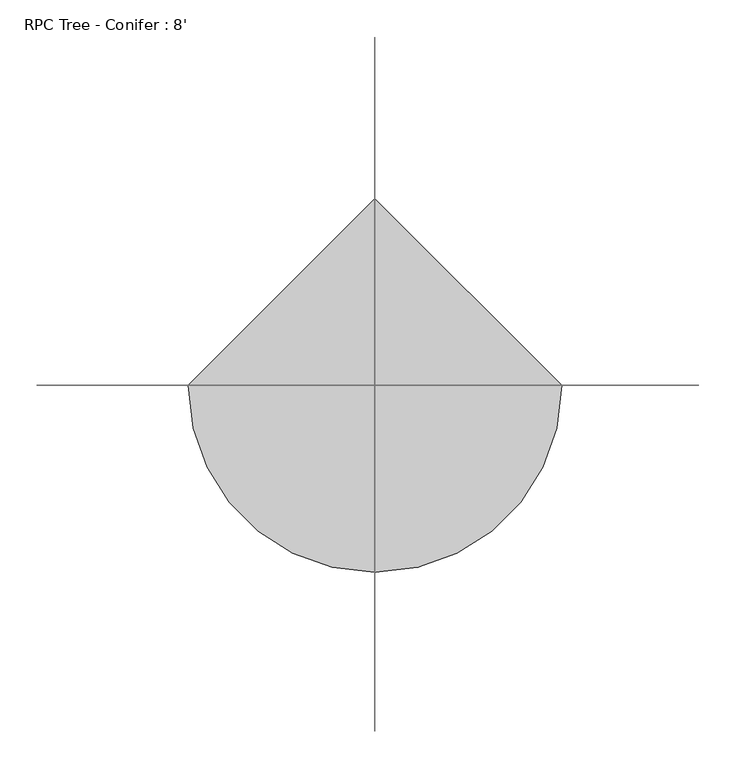
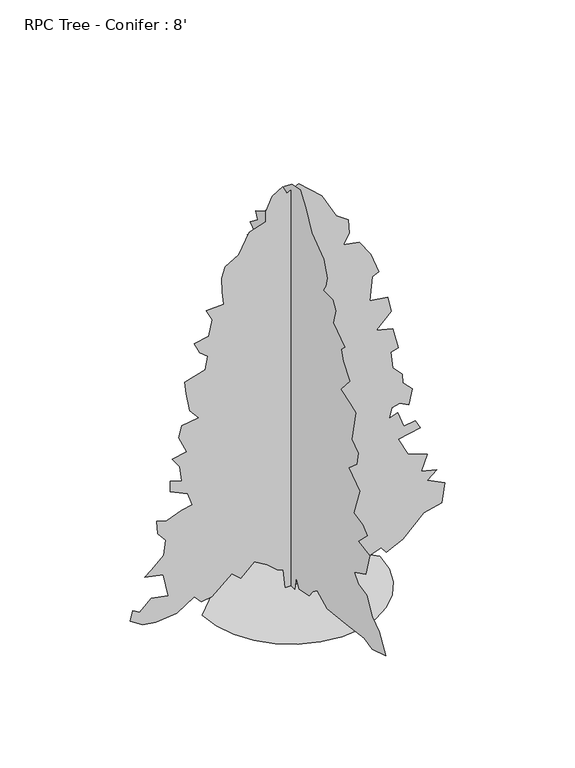
"""IFC4 building model written with IfcOpenShell, lengths in millimetres: geographic element geometry, RPC Tree - Conifer : 8'."""

from ifc_helpers import new_model, si_unit, origin, place, context, project, spatial, triangles, source, transform, mapped, element, save


def rpc_tree_conifer_8_e62f4ae5(model_context):
    return source(origin(), model_context, "Body", "Tessellation", [
        triangles([(0.1966718, 15.1865072, 1.1e-05), (0.196674, 23.4382814, 63.9513063), (0.1966753, 33.7530179, 92.8321697), (0.1966764, 70.8859666, 72.2030828), (0.1966779, 116.2705283, 53.6365698), (0.1966799, 167.8442245, 45.3847979), (0.1966823, 219.5611622, 47.5799673), (0.1966815, 225.6068687, 12.3776999), (0.1966839, 262.7398856, 37.1330214), (0.1966849, 302.1406238, 11.0749077), (0.1966865, 330.8169803, 20.629473), (0.1966889, 386.5168871, 18.5665107), (0.1966909, 413.3346906, 43.3218333), (0.1966951, 471.0973712, 99.0211361), (0.196694, 436.0270555, 115.5245346), (0.1966929, 405.083014, 125.8397299), (0.1966916, 376.2588286, 123.43181), (0.1966923, 370.0127346, 156.7837804), (0.1966935, 378.2644112, 185.6651025), (0.1966958, 407.1457515, 218.6718996), (0.1966947, 378.2644112, 224.860875), (0.1966963, 400.956776, 245.4904843), (0.1966951, 365.8872597, 255.8049165), (0.196694, 328.7542428, 274.3718246), (0.1966942, 309.6630753, 312.5739078), (0.1966968, 357.6355468, 325.9455116), (0.1966983, 378.2644112, 344.5116385), (0.1966972, 351.4466077, 350.7005776), (0.196696, 306.0618779, 377.5191805), (0.196698, 339.0686568, 394.0225699), (0.1966997, 341.7386973, 448.3478514), (0.1966982, 303.9983774, 453.8479517), (0.196697, 270.9915803, 462.0996646), (0.1966983, 275.8607599, 499.6875956), (0.1967004, 316.0593055, 511.0192803), (0.196702, 324.6280048, 550.8063503), (0.1967003, 291.6212078, 544.6174112), (0.1967006, 270.7766952, 584.7671771), (0.1967025, 293.6839452, 612.6945059), (0.1967019, 264.8026231, 637.4496082), (0.1967038, 293.6839452, 658.0792356), (0.1967047, 301.93564, 674.5825888), (0.1967034, 250.3619529, 707.590167), (0.1967037, 244.1729957, 728.2189951), (0.1967061, 285.4322505, 748.8486225), (0.1967061, 266.8653605, 775.6703138), (0.1967048, 225.6068687, 794.2326256), (0.196707, 252.4246904, 825.1773937), (0.1967065, 223.5433682, 851.9921814), (0.1967056, 186.4111144, 878.8145994), (0.1967065, 184.3476139, 911.8244305), (0.1967083, 215.2916735, 926.2643194), (0.1967078, 192.6000717, 942.7692713), (0.1967068, 165.781487, 948.9566843), (0.1967091, 200.8517664, 973.7064817), (0.1967083, 163.7187495, 1002.59389), (0.1967094, 174.0331817, 1023.221192), (0.1967082, 130.7111985, 1047.9786198), (0.1967077, 95.64091, 1085.1108736), (0.1967081, 72.5007936, 1132.743504), (0.1967077, 29.6270933, 1184.1327364), (0.196707, -3.3800643, 1210.9475241), (0.1967054, -44.6389495, 1219.2), (0.196703, -73.520199, 1182.0677462), (0.1967, -102.4013713, 1124.3081177), (0.196696, -162.2267439, 1080.9808205), (0.1966939, -178.7301516, 1033.5387308), (0.1966934, -170.4784568, 1004.6512499), (0.1966933, -160.1640246, 986.0889381), (0.1966913, -205.5487362, 986.0889381), (0.1966899, -219.9894064, 961.331583), (0.1966892, -207.6114737, 918.0119162), (0.1966854, -265.374118, 878.8145994), (0.1966857, -246.807228, 862.3096476), (0.1966844, -257.1224233, 831.3648794), (0.1966817, -290.1292203, 792.1675627), (0.1966822, -244.7444906, 740.596946), (0.1966796, -292.5295099, 725.6693687), (0.1966781, -319.0105425, 713.7791061), (0.1966762, -300.4436525, 623.0089199), (0.1966742, -331.388457, 600.316555), (0.1966733, -325.1995179, 563.1835382), (0.196674, -286.0029824, 528.1140218), (0.1966705, -339.6401699, 490.9809686), (0.1966694, -308.6960921, 406.3997578), (0.1966671, -354.0808219, 398.1480449), (0.1966656, -376.7731868, 379.581918), (0.1966662, -331.388457, 334.1971882), (0.1966634, -389.1503383, 325.9455116), (0.1966623, -368.5214739, 257.8676539), (0.196664, -312.8215671, 231.0498323), (0.1966624, -331.388457, 206.2947299), (0.1966602, -374.7096863, 198.0430352), (0.1966576, -401.5282891, 150.5948231), (0.1966553, -436.5985685, 125.8397299), (0.1966523, -467.54261, 72.2030828), (0.1966547, -401.5282891, 51.5736098), (0.1966568, -361.0409348, 60.8274872), (0.1966604, -272.9468752, 50.0099062), (0.1966643, -178.7301516, 39.1959088), (0.1966672, -129.219202, 63.9513063), (0.1966676, -108.5903376, 47.4476807), (0.1966678, -90.0234386, 24.7553226), (0.1966697, -40.513025, 14.4406622), (0.1966711, -26.1805672, 40.634947), (0.1966703, -17.8206657, 1e-05), (-15.4704299, 4e-07, 1.1e-05), (-21.659243, -6.3e-06, 55.6995344), (-38.1627869, -6.1e-06, 61.8883463), (-67.0440363, -6.4e-06, 86.6439755), (-104.1767534, -6.3e-06, 109.3363313), (-143.3732708, 1e-06, 72.2030828), (-168.1283823, 7e-07, 94.8956702), (-225.8910265, 4.6e-06, 45.3847979), (-254.8965599, 5.7e-06, 41.7547052), (-275.4012131, 5.3e-06, 63.9513063), (-324.9121445, 8.2e-06, 30.9442095), (-384.7375262, 1.47e-05, 24.7553998), (-421.8705431, 1.56e-05, 30.9442095), (-456.9408225, 1.56e-05, 53.6365698), (-450.7518834, 1.41e-05, 82.5177376), (-430.122256, 1.4e-05, 70.1401183), (-397.1146777, 7.3e-06, 101.0846366), (-349.6672468, 6.2e-06, 92.8321697), (-363.659852, 3.6e-06, 160.9686812), (-415.6815677, 4.7e-06, 171.2244505), (-397.1146777, 3.5e-06, 185.6651025), (-362.0451613, 1e-06, 218.6718996), (-355.8561859, -1.2e-06, 261.9938919), (-378.5485508, -1.7e-06, 288.8124766), (-382.6747888, -3.3e-06, 328.0082491), (-353.7934848, -3.8e-06, 319.7565362), (-310.4714925, -1.03e-05, 336.2599257), (-281.5901703, -1.14e-05, 342.4489011), (-293.968103, -1.27e-05, 379.581918), (-343.5224547, -1.23e-05, 402.7909301), (-343.4782714, -1.37e-05, 435.2810617), (-310.4714925, -1.42e-05, 424.9666477), (-316.0379042, -1.6e-05, 468.8151704), (-337.290059, -1.68e-05, 499.2326815), (-296.0308405, -1.84e-05, 507.4843944), (-318.723169, -1.99e-05, 556.9945627), (-310.4714925, -2.16e-05, 590.0021047), (-263.0240434, -2.78e-05, 598.2538176), (-287.7791458, -2.84e-05, 627.1351215), (-298.093578, -3.06e-05, 682.8342653), (-302.2197978, -3.2e-05, 717.9045811), (-244.4571535, -3.46e-05, 736.4707443), (-236.2054587, -3.65e-05, 773.6052509), (-258.8978236, -3.66e-05, 792.1675627), (-275.4012131, -3.76e-05, 825.1773937), (-233.4508304, -4.36e-05, 832.2411341), (-223.827526, -4.6e-05, 878.8145994), (-240.3309155, -4.69e-05, 911.8244305), (-190.820729, -4.85e-05, 913.881863), (-194.9462039, -5.01e-05, 953.0791071), (-197.0097044, -5.19e-05, 994.3414141), (-186.6945092, -5.36e-05, 1025.2862549), (-148.4565725, -6.02e-05, 1048.7939043), (-118.6174145, -6.37e-05, 1105.7381756), (-71.1698837, -6.57e-05, 1120.1780645), (-71.1698837, -6.71e-05, 1151.1229053), (-52.6033753, -6.94e-05, 1190.3202221), (-23.7222053, -7.11e-05, 1208.8825338), (-11.3445042, -7.05e-05, 1186.190169), (21.6625903, -7.66e-05, 1202.6950481), (87.6765615, -7.59e-05, 1142.8704294), (128.9358072, -6.94e-05, 1068.6059217), (164.0060866, -7.37e-05, 1043.8485666), (166.0688241, -6.75e-05, 1002.59389), (149.5654346, -6.58e-05, 973.7064817), (194.9501462, -6.67e-05, 965.4616362), (227.9569433, -6.56e-05, 918.0119162), (250.6493082, -6.36e-05, 858.1872248), (231.8827575, -6.26e-05, 848.4260473), (223.8314684, -5.93e-05, 779.792664), (275.4043924, -6.05e-05, 771.5402607), (285.7195876, -5.87e-05, 726.1562576), (242.3975953, -5.56e-05, 684.8978022), (289.8450625, -5.65e-05, 672.5198513), (306.349215, -4.97e-05, 608.5682679), (283.6560871, -4.88e-05, 604.442793), (289.8450625, -4.68e-05, 554.9318253), (317.1269729, -4.63e-05, 525.1307736), (318.7264029, -4.52e-05, 499.2326815), (345.5449694, -4.48e-05, 472.4140786), (335.2297923, -4.24e-05, 427.0293852), (310.47469, -4.23e-05, 441.4700372), (287.7823251, -4.14e-05, 435.2810617), (279.5306304, -3.98e-05, 406.3997578), (304.2857145, -4.09e-05, 414.6514343), (320.7891403, -3.93e-05, 367.2040034), (353.7966823, -4.06e-05, 373.3929425), (368.2373343, -3.98e-05, 346.574376), (306.349215, -3.74e-05, 334.1971882), (333.1670548, -3.14e-05, 280.5600188), (388.8669617, -3.66e-05, 259.9311544), (371.0430133, -2.96e-05, 214.5471877), (415.6848015, -3.04e-05, 204.2312476), (388.8669617, -2.86e-05, 181.5388827), (438.3771664, -2.9e-05, 156.7837804), (430.1254535, -2.62e-05, 99.0211361), (378.5517846, -2.41e-05, 86.6439755), (319.0098521, -1.97e-05, 28.7259515), (271.2789175, -1.28e-05, 6.1888114), (256.8382655, -1.32e-05, 24.7553226), (202.687501, -1.08e-05, 6.3862074), (145.4392058, -9e-06, 4.1258794), (122.74685, -9.3e-06, 24.7553226), (71.1732401, -8.5e-06, 43.3218333), (22.4985813, -6.6e-06, 33.3508349), (17.5366669, -5e-06, 1.01e-05), (-252.3080369, -1.4e-06, 1.81e-05), (-245.6321544, -57.8572879, 1.62e-05), (-226.6210147, -110.9898732, 1.4e-05), (-196.7955823, -157.8757377, 1.17e-05), (-157.6790746, -196.9922454, 9.4e-06), (-110.793201, -226.8176778, 7.1e-06), (-57.6606156, -245.8288176, 5e-06), (0.1966821, -252.5047, 3.1e-06), (58.0539601, -245.8288176, 1.5e-06), (111.1865454, -226.8176778, 5e-07), (158.0724009, -196.9922454, 0.0), (197.1889086, -157.8757377, 0.0), (227.014341, -110.9898732, 5e-07), (246.0254807, -57.8572879, 1.5e-06), (252.7013632, 2.34e-05, 3.1e-06), (0.196638, 252.5047, 1.81e-05)], [[26, 27, 28], [21, 22, 23], [19, 20, 21], [51, 52, 53], [7, 8, 9], [35, 36, 37], [13, 14, 15], [34, 35, 37], [54, 55, 56], [72, 73, 74], [95, 96, 97], [88, 89, 90], [44, 45, 46], [86, 87, 88], [85, 86, 88], [51, 53, 54], [44, 46, 47], [88, 90, 91], [13, 15, 16], [13, 16, 17], [38, 39, 40], [25, 26, 28], [25, 28, 29], [47, 48, 49], [56, 57, 58], [30, 31, 32], [29, 30, 32], [41, 42, 43], [40, 41, 43], [106, 1, 2], [105, 106, 2], [75, 76, 77], [94, 95, 97], [94, 97, 98], [78, 79, 80], [83, 84, 85], [29, 32, 33], [103, 104, 105], [12, 13, 17], [11, 12, 17], [77, 78, 80], [102, 103, 105], [62, 63, 64], [80, 81, 82], [80, 82, 83], [61, 62, 64], [61, 64, 65], [60, 61, 65], [59, 60, 65], [69, 70, 71], [69, 71, 72], [94, 98, 99], [93, 94, 99], [92, 93, 99], [92, 99, 100], [91, 92, 100], [91, 100, 101], [47, 49, 50], [9, 10, 11], [9, 11, 17], [9, 17, 18], [7, 9, 18], [59, 65, 66], [59, 66, 67], [59, 67, 68], [59, 68, 69], [58, 59, 69], [56, 58, 69], [54, 56, 69], [54, 69, 72], [51, 54, 72], [50, 51, 72], [50, 72, 74], [50, 74, 75], [50, 75, 77], [47, 50, 77], [44, 47, 77], [43, 44, 77], [40, 43, 77], [40, 77, 80], [40, 80, 83], [38, 40, 83], [38, 83, 85], [37, 38, 85], [34, 37, 85], [33, 34, 85], [29, 33, 85], [25, 29, 85], [25, 85, 88], [25, 88, 91], [25, 91, 101], [25, 101, 102], [24, 25, 102], [23, 24, 102], [21, 23, 102], [105, 2, 3], [102, 105, 3], [21, 102, 3], [21, 3, 4], [21, 4, 5], [21, 5, 6], [21, 6, 7], [21, 7, 18], [19, 21, 18], [125, 126, 127], [198, 199, 200], [153, 154, 155], [139, 140, 141], [130, 131, 132], [120, 121, 122], [119, 120, 122], [186, 187, 188], [136, 137, 138], [135, 136, 138], [150, 151, 152], [193, 194, 195], [192, 193, 195], [125, 127, 128], [180, 181, 182], [163, 164, 165], [185, 186, 188], [196, 197, 198], [190, 191, 192], [111, 112, 113], [212, 107, 108], [211, 212, 108], [173, 174, 175], [149, 150, 152], [179, 180, 182], [129, 130, 132], [146, 147, 148], [204, 205, 206], [200, 201, 202], [200, 202, 203], [162, 163, 165], [190, 192, 195], [165, 166, 167], [118, 119, 122], [118, 122, 123], [118, 123, 124], [117, 118, 124], [116, 117, 124], [176, 177, 178], [176, 178, 179], [129, 132, 133], [185, 188, 189], [142, 143, 144], [141, 142, 144], [161, 162, 165], [161, 165, 167], [161, 167, 168], [116, 124, 125], [145, 146, 148], [144, 145, 148], [114, 115, 116], [113, 114, 116], [113, 116, 125], [113, 125, 128], [113, 128, 129], [113, 129, 133], [113, 133, 134], [111, 113, 134], [168, 169, 170], [168, 170, 171], [161, 168, 171], [160, 161, 171], [159, 160, 171], [158, 159, 171], [157, 158, 171], [156, 157, 171], [155, 156, 171], [171, 172, 173], [171, 173, 175], [155, 171, 175], [155, 175, 176], [153, 155, 176], [152, 153, 176], [149, 152, 176], [149, 176, 179], [148, 149, 179], [144, 148, 179], [144, 179, 182], [144, 182, 183], [141, 144, 183], [139, 141, 183], [138, 139, 183], [135, 138, 183], [134, 135, 183], [111, 134, 183], [110, 111, 183], [110, 183, 184], [110, 184, 185], [110, 185, 189], [110, 189, 190], [110, 190, 195], [109, 110, 195], [108, 109, 195], [211, 108, 195], [210, 211, 195], [210, 195, 196], [209, 210, 196], [209, 196, 198], [208, 209, 198], [207, 208, 198], [206, 207, 198], [204, 206, 198], [203, 204, 198], [200, 203, 198], [227, 228, 213], [226, 227, 213], [226, 213, 214], [225, 226, 214], [225, 214, 215], [225, 215, 216], [224, 225, 216], [223, 224, 216], [223, 216, 217], [223, 217, 218], [223, 218, 219], [223, 219, 220], [223, 220, 221], [223, 221, 222]], closed=False),
    ])


if __name__ == "__main__":
    model = new_model("IFC4")
    model_context = context("Model", 3, world=origin())
    ifc_project = project(units=[si_unit("LENGTHUNIT", "METRE", prefix="MILLI")], contexts=[model_context])
    site = spatial("IfcSite", under=ifc_project)
    building = spatial("IfcBuilding", under=site)
    placement = place(None, origin())
    rpc_tree_conifer_8_shape = rpc_tree_conifer_8_e62f4ae5(model_context)
    element("IfcGeographicElement", 1, ObjectType="RPC Tree - Conifer : 8'", at=placement, inside=building, context=model_context, shape_type="MappedRepresentation", body=[
        mapped(rpc_tree_conifer_8_shape, transform((0.0, 0.0, 0.0), x_axis=(1.0, 0.0, 0.0), y_axis=(0.0, 1.0, 0.0), z_axis=(0.0, 0.0, 1.0))),
    ])
    save(model, "model.ifc")

# Revit data of these elements
# Type "RPC Tree - Conifer : 8'"
#   built-in parameter 1005198 = "{2, 15},{39, RPC-16-G0M4-N9PX-U6TN-C000-ST1L-LVER-AU},{1, 0},{1, 0},{2, 13},{1, 8},{5, Color},{1, 0},{1, 0},{3, 0.8},{3, 0.8},{3, 0.8},{1, 8},{7, BBoxMin},{1, 0},{1, 0},{1, 0},{1, 0},{1, 0},{1, 8},{7, BBoxMax},{1, 0},{1, 0},{1, 0},{1, 0},{1, 0},{2, 11},{9, RPCTypeId},{1, 0},{1, 0},{39, RPC-16-G0M4-N9PX-U6TN-C000-ST1L-LVER-AU},{1, 6},{14, RPCPlantHeight},{1, 0},{1, 0},{2, 13},{2, 11},{7, keyword},{1, 0},{1, 0},{34, :RPCs:Trees [General]:Geometry:RPC},{2, 11},{8, category},{1, 0},{1, 0},{15, Trees [General]},{2, 11},{12, LocalizedUID},{1, 0},{1, 0},{15, Colorado Spruce},{2, 14},{6, Height},{1, 0},{1, 0},{2, 13},{1, 2},{16, Cast Reflections},{1, 0},{1, 0},{1, 0},{1, 2},{12, Cast Shadows},{1, 0},{1, 0},{1, 1},{1, 2},{9, Lock View},{1, 0},{1, 0},{1, 0},{1, 4},{5, ViewC},{1, 0},{1, 0},{1, 0},{21, assetlibrary_base.fbx},{1, 5},"
#   built-in parameter 1005195 = "RPC-16-G0M4-N9PX-U6TN-C000-ST1L-LVER-AU"
#   Assembly Code = "G2050500"
#   Height = 4' - 0"
#   Description = (empty or 0)
#   Default Elevation = 0
